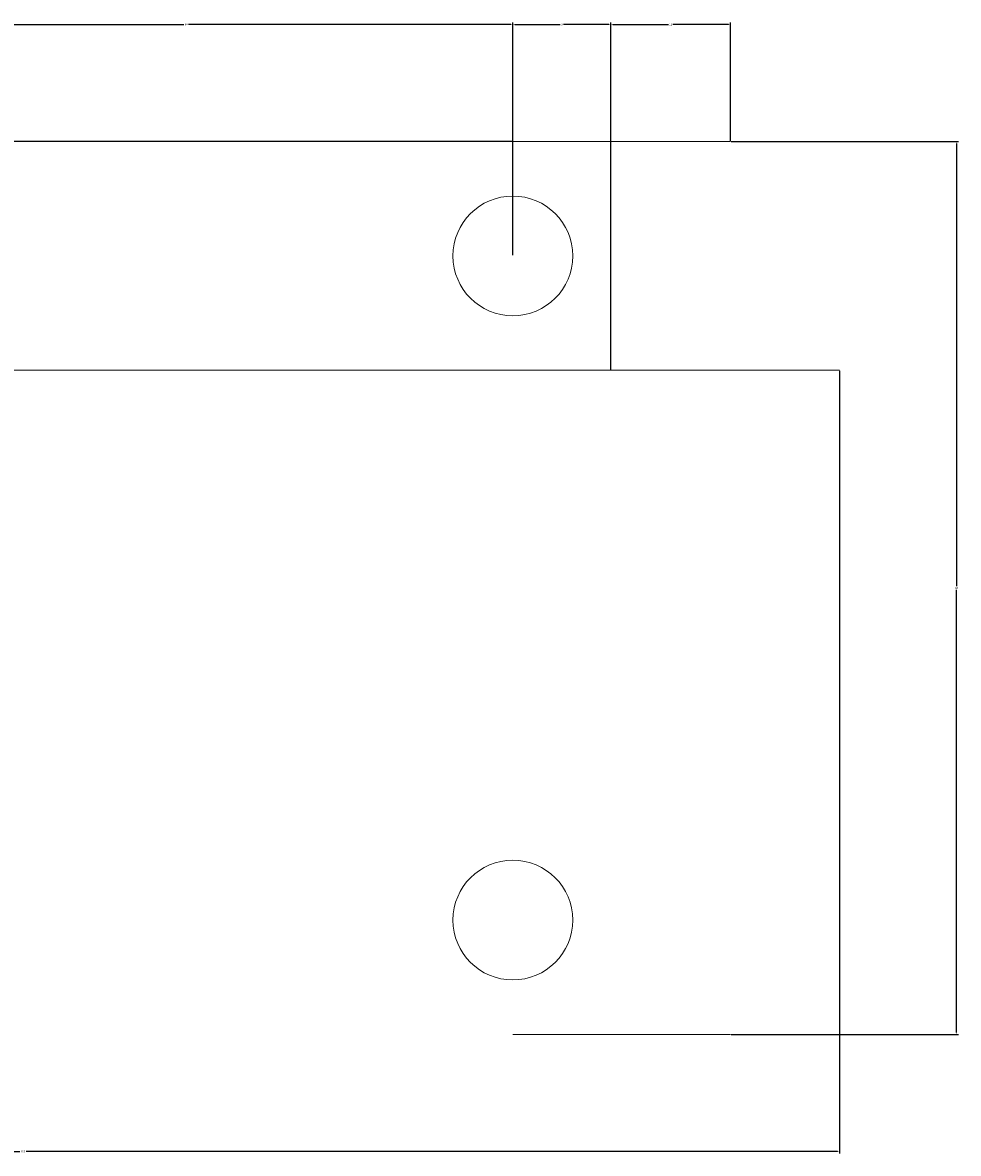
# Model space of a CAD drawing. Units: millimetres. Extents: x 315 to 487, y -72 to 32.
# Tile 4 of 4: x 401 to 487, y -72 to 32. Entities that reach past the tile are written whole.
import ezdxf

# ---------------------------------------------------------------- set-up
doc = ezdxf.new("R2010")
doc.units = ezdxf.units.MM
doc.layers.add('M-CONS', color=8, linetype='Continuous', lineweight=13)
doc.layers.add('M-DIMS', color=2, linetype='Continuous', lineweight=18)
doc.styles.get("Standard").update_dxf_attribs({"font": 'arial.ttf'})
doc.dimstyles.get("Standard").update_dxf_attribs({"dimtxt": 0.18, "dimasz": 0.18, "dimexe": 0.18, "dimexo": 0.0625, "dimgap": 0.09, "dimtad": 0, "dimtih": 1, "dimtoh": 1, "dimdec": 4, "dimzin": 0, "dimdsep": 46, "dimtxsty": 'Standard', "dimcen": 0.09, "dimadec": 0, "dimazin": 0, "dimtfac": 1, "dimtdec": 4, "dimtofl": 0, "dimtmove": 0, "dimatfit": 3, "dimfxl": 1, "dimtolj": 1, "dimtzin": 0, "dimarcsym": 0})

# ---------------------------------------------------------------- blocks, each defined once
blk = doc.blocks.new('*D3')
at = {"layer": 'Defpoints', "color": 0, "transparency": 16777216}
for p in [(326.01, 0), (476.01, 0), (476.01, -71.75)]:
    blk.add_point(p, dxfattribs=at)
at = {"layer": 'M-DIMS', "color": 0, "lineweight": -2, "transparency": 16777216}
for p, q in [((326.01, -0.06), (326.01, -71.93)), ((476.01, -0.06), (476.01, -71.93)), ((326.19, -71.75), (400.73, -71.75)), ((475.83, -71.75), (401.29, -71.75))]:
    blk.add_line(p, q, dxfattribs=at)
at = {"layer": 'M-DIMS', "color": 0, "transparency": 16777216}
for points in [[(326.19, -71.72), (326.19, -71.78), (326.01, -71.75)], [(475.83, -71.72), (475.83, -71.78), (476.01, -71.75)]]:
    blk.add_solid(points, dxfattribs=at)
at = {"layer": 'M-DIMS', "color": 0, "transparency": 16777216, "insert": (401.01, -71.75), "char_height": 0.18, "attachment_point": 5}
blk.add_mtext('\\A1;150', dxfattribs=at)
blk = doc.blocks.new('*D4')
at = {"layer": 'Defpoints', "color": 0, "transparency": 16777216}
for p in [(466.01, 21), (486.76, 21), (466.01, -61)]:
    blk.add_point(p, dxfattribs=at)
at = {"layer": 'M-DIMS', "color": 0, "lineweight": -2, "transparency": 16777216}
for p, q in [((466.07, 21), (486.94, 21)), ((486.76, 20.82), (486.76, -19.82)), ((486.76, -60.82), (486.76, -20.18)), ((466.07, -61), (486.94, -61))]:
    blk.add_line(p, q, dxfattribs=at)
at = {"layer": 'M-DIMS', "color": 0, "transparency": 16777216}
for points in [[(486.73, 20.82), (486.79, 20.82), (486.76, 21)], [(486.73, -60.82), (486.79, -60.82), (486.76, -61)]]:
    blk.add_solid(points, dxfattribs=at)
at = {"layer": 'M-DIMS', "color": 0, "transparency": 16777216, "insert": (486.76, -20), "char_height": 0.18, "attachment_point": 5}
blk.add_mtext('\\A1;82', dxfattribs=at)
blk = doc.blocks.new('*D7')
at = {"layer": 'Defpoints', "color": 0, "transparency": 16777216}
for p in [(446.01, 31.75), (386.01, 10.5), (446.01, 10.5)]:
    blk.add_point(p, dxfattribs=at)
at = {"layer": 'M-DIMS', "color": 0, "lineweight": -2, "transparency": 16777216}
for p, q in [((386.01, 10.56), (386.01, 31.93)), ((386.19, 31.75), (415.79, 31.75)), ((445.83, 31.75), (416.23, 31.75)), ((446.01, 10.56), (446.01, 31.93))]:
    blk.add_line(p, q, dxfattribs=at)
at = {"layer": 'M-DIMS', "color": 0, "transparency": 16777216}
for points in [[(386.19, 31.78), (386.19, 31.72), (386.01, 31.75)], [(445.83, 31.78), (445.83, 31.72), (446.01, 31.75)]]:
    blk.add_solid(points, dxfattribs=at)
at = {"layer": 'M-DIMS', "color": 0, "transparency": 16777216, "insert": (416.01, 31.75), "char_height": 0.18, "attachment_point": 5}
blk.add_mtext('\\A1;60', dxfattribs=at)
blk = doc.blocks.new('*D8')
at = {"layer": 'Defpoints', "color": 0, "transparency": 16777216}
for p in [(455.01, 31.75), (446.01, 10.5), (455.01, 0)]:
    blk.add_point(p, dxfattribs=at)
at = {"layer": 'M-DIMS', "color": 0, "lineweight": -2, "transparency": 16777216}
for p, q in [((446.01, 10.56), (446.01, 31.93)), ((446.19, 31.75), (450.36, 31.75)), ((454.83, 31.75), (450.66, 31.75)), ((455.01, 0.06), (455.01, 31.93))]:
    blk.add_line(p, q, dxfattribs=at)
at = {"layer": 'M-DIMS', "color": 0, "transparency": 16777216}
for points in [[(446.19, 31.78), (446.19, 31.72), (446.01, 31.75)], [(454.83, 31.78), (454.83, 31.72), (455.01, 31.75)]]:
    blk.add_solid(points, dxfattribs=at)
at = {"layer": 'M-DIMS', "color": 0, "transparency": 16777216, "insert": (450.51, 31.75), "char_height": 0.18, "attachment_point": 5}
blk.add_mtext('\\A1;9', dxfattribs=at)
blk = doc.blocks.new('*D9')
at = {"layer": 'Defpoints', "color": 0, "transparency": 16777216}
for p in [(466.01, 31.75), (466.01, 21), (455.01, 0)]:
    blk.add_point(p, dxfattribs=at)
at = {"layer": 'M-DIMS', "color": 0, "lineweight": -2, "transparency": 16777216}
for p, q in [((455.01, 0.06), (455.01, 31.93)), ((455.19, 31.75), (460.31, 31.75)), ((465.83, 31.75), (460.7, 31.75)), ((466.01, 21.06), (466.01, 31.93))]:
    blk.add_line(p, q, dxfattribs=at)
at = {"layer": 'M-DIMS', "color": 0, "transparency": 16777216}
for points in [[(455.19, 31.78), (455.19, 31.72), (455.01, 31.75)], [(465.83, 31.78), (465.83, 31.72), (466.01, 31.75)]]:
    blk.add_solid(points, dxfattribs=at)
at = {"layer": 'M-DIMS', "color": 0, "transparency": 16777216, "insert": (460.51, 31.75), "char_height": 0.18, "attachment_point": 5}
blk.add_mtext('\\A1;11', dxfattribs=at)
blk = doc.blocks.new('*D12')
at = {"layer": 'Defpoints', "color": 0, "transparency": 16777216}
for p in [(315.26, 21), (446.01, 21), (386.01, 10.5)]:
    blk.add_point(p, dxfattribs=at)
at = {"layer": 'M-DIMS', "color": 0, "lineweight": -2, "transparency": 16777216}
for p, q in [((445.94, 21), (315.08, 21)), ((315.26, 20.82), (315.26, 15.93)), ((315.26, 10.68), (315.26, 15.57)), ((385.94, 10.5), (315.08, 10.5))]:
    blk.add_line(p, q, dxfattribs=at)
at = {"layer": 'M-DIMS', "color": 0, "transparency": 16777216}
for points in [[(315.23, 20.82), (315.29, 20.82), (315.26, 21)], [(315.23, 10.68), (315.29, 10.68), (315.26, 10.5)]]:
    blk.add_solid(points, dxfattribs=at)
at = {"layer": 'M-DIMS', "color": 0, "transparency": 16777216, "insert": (315.26, 15.75), "char_height": 0.18, "attachment_point": 5}
blk.add_mtext('\\A1;10.5', dxfattribs=at)

msp = doc.modelspace()

# ---------------------------------------------------------------- linework, layer by layer
at = {"layer": 'M-CONS'}
for p, q in [((466.01, 21, 200.05), (446.01, 21, 200.05)), ((466.01, -61, 200.05), (446.01, -61, 200.05))]:
    msp.add_line(p, q, dxfattribs=at)
at = {"layer": 'M-CONS', "extrusion": (0, -1, 0)}
for p, q in [((326.01, 0, 190.05), (476.01, 0, 190.05)), ((466.01, 0, 200.05), (326.01, 0, 200.05)), ((434.01, 0, 240.05), (338.27, 0, 222.3)), ((434.01, 0, 261.07), (434.01, 0, 240.05)), ((476.01, 0, 190.05), (446.01, 0, 190.07)), ((466.01, 0, 232.05), (466.01, 0, 200.05)), ((476.01, 0, 235.05), (469.01, 0, 235.05)), ((476.01, 0, 190.05), (476.01, 0, 235.05)), ((476.01, 0, 235.05), (476.01, 0, 261.07))]:
    msp.add_line(p, q, dxfattribs=at)
at = {"layer": 'M-CONS'}
for centre in [(446.01, 10.5, 200.05), (446.01, -50.5, 200.05)]:
    msp.add_circle(centre, 5.5, dxfattribs=at)
at = {"layer": 'M-CONS', "extrusion": (0, -1, 0)}
msp.add_circle((455.01, 261.07), 8, dxfattribs=at)
for centre, radius, start in [((455.01, 261.07), 21, 0), ((469.01, 232.05), 3, 90)]:
    msp.add_arc(centre, radius, start, 180, dxfattribs=at)

# ---------------------------------------------------------------- dimensions: what is measured, and where the dimension line sits
at = {"layer": 'M-DIMS'}
for base, p1, p2, picture, middle in [((446.01, 31.75), (386.01, 10.5), (446.01, 10.5), '*D7', (416.01, 31.75)), ((455.01, 31.75), (446.01, 10.5), (455.01, 0), '*D8', (450.51, 31.75)), ((466.01, 31.75), (455.01, 0), (466.01, 21), '*D9', (460.51, 31.75)), ((476.01, -71.75), (326.01, 0), (476.01, 0), '*D3', (401.01, -71.75))]:
    dim = msp.add_linear_dim(base=base, p1=p1, p2=p2, dimstyle='Standard', override={"dimdec": 0, "dimlfac": 1, "dimrnd": 0, "dimzin": 0, "dimdsep": 46, "dimlunit": 2}, dxfattribs=at)
    dim.commit()
    dim.dimension.update_dxf_attribs({"geometry": picture, "text_midpoint": middle})
for base, p1, p2, override, picture, middle in [((315.26, 21), (386.01, 10.5), (446.01, 21), {"dimdec": 1, "dimlfac": 1, "dimrnd": 0, "dimzin": 0, "dimdsep": 46, "dimlunit": 2}, '*D12', (315.26, 15.75)), ((486.76, 21), (466.01, -61), (466.01, 21), {"dimdec": 0, "dimlfac": 1, "dimrnd": 0, "dimzin": 0, "dimdsep": 46, "dimlunit": 2}, '*D4', (486.76, -20))]:
    dim = msp.add_linear_dim(base=base, p1=p1, p2=p2, angle=90, dimstyle='Standard', override=override, dxfattribs=at)
    dim.commit()
    dim.dimension.update_dxf_attribs({"geometry": picture, "text_midpoint": middle})

doc.saveas('drawing.dxf')
